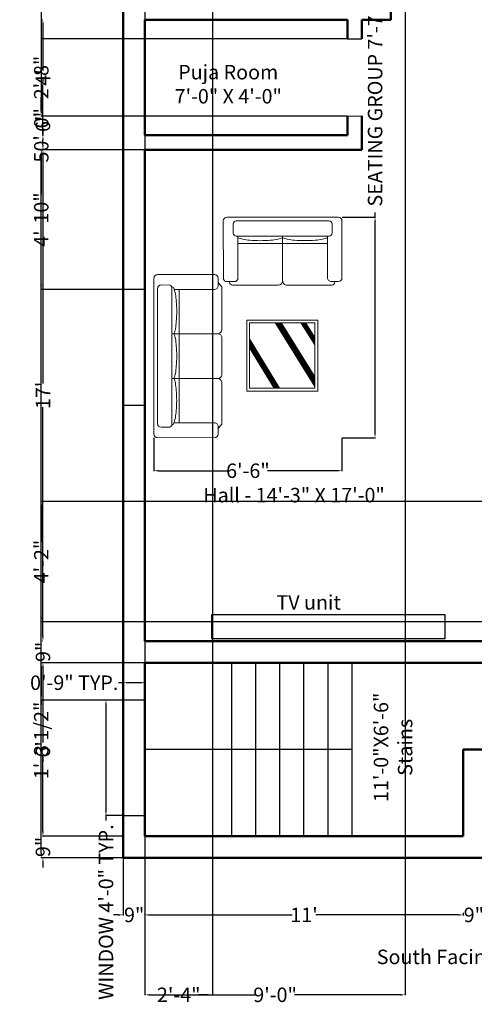
# Model space of a CAD drawing. Units: inches. Extents: x 35 to 505, y 81 to 785.
# Tile 1 of 3: x 35 to 224, y 86 to 495. Entities that reach past the tile are written whole.
import ezdxf

# ---------------------------------------------------------------- set-up
doc = ezdxf.new("R2010")
doc.units = ezdxf.units.IN
doc.header["$MEASUREMENT"] = 0
for name, color, linetype, lineweight in [('A-ANNO-DIMS', 2, 'Continuous', 13), ('A-ANNO-TEXT', 7, 'Continuous', 18), ('A-AREA-IDEN', 7, 'Continuous', 20), ('A-DOOR', 3, 'Continuous', 30), ('A-FLOR-CASE', 8, 'Continuous', 25), ('A-FLOR-STRS', 7, 'Continuous', 25), ('A-FURN', 6, 'Continuous', 18), ('A-GLAZ', 4, 'Continuous', 25), ('A-WALL', 7, 'Continuous', 50)]:
    doc.layers.add(name, color=color, linetype=linetype, lineweight=lineweight)
doc.styles.get("Standard").update_dxf_attribs({"font": 'arial.ttf'})
doc.dimstyles.get("Standard").update_dxf_attribs({"dimtxt": 6, "dimasz": 2, "dimexe": 0.18, "dimexo": 0.0625, "dimgap": 0.09, "dimtad": 0, "dimdec": 0, "dimzin": 0, "dimdsep": 46, "dimlunit": 4, "dimtxsty": 'Standard', "dimcen": 0.09, "dimadec": 0, "dimazin": 0, "dimtfac": 1, "dimtdec": 0, "dimtofl": 0, "dimtmove": 0, "dimatfit": 3, "dimfxl": 1, "dimtolj": 1, "dimtzin": 0, "dimarcsym": 0})

# ---------------------------------------------------------------- blocks, each defined once
blk = doc.blocks.new('*D1')
at = {"layer": 'A-ANNO-DIMS', "color": 0, "lineweight": -2, "transparency": 16777216}
for p, q in [((44.71, 158.11), (44.71, 160.11)), ((77.99, 156.11), (44.53, 156.11)), ((44.65, 147.11), (44.53, 147.11)), ((44.71, 145.11), (44.71, 143.11))]:
    blk.add_line(p, q, dxfattribs=at)
at = {"layer": 'A-ANNO-DIMS', "color": 0, "transparency": 16777216}
for points in [[(44.38, 158.11), (45.04, 158.11), (44.71, 156.11)], [(44.38, 145.11), (45.04, 145.11), (44.71, 147.11)]]:
    blk.add_solid(points, dxfattribs=at)
at = {"layer": 'Defpoints', "color": 0, "transparency": 16777216}
for p in [(44.71, 156.11), (78.06, 156.11), (44.71, 147.11)]:
    blk.add_point(p, dxfattribs=at)
at = {"layer": 'A-ANNO-DIMS', "color": 0, "transparency": 16777216, "insert": (44.71, 151.61), "char_height": 6, "attachment_point": 5, "rotation": 90}
blk.add_mtext('\\A1;9"', dxfattribs=at)
blk = doc.blocks.new('*D2')
at = {"layer": 'A-ANNO-DIMS', "color": 0, "lineweight": -2, "transparency": 16777216}
for p, q in [((44.65, 228.11), (44.53, 228.11)), ((44.71, 226.11), (44.71, 194.98)), ((44.71, 158.11), (44.71, 189.24)), ((44.77, 156.11), (44.89, 156.11))]:
    blk.add_line(p, q, dxfattribs=at)
at = {"layer": 'A-ANNO-DIMS', "color": 0, "transparency": 16777216}
for points in [[(44.38, 226.11), (45.04, 226.11), (44.71, 228.11)], [(44.38, 158.11), (45.04, 158.11), (44.71, 156.11)]]:
    blk.add_solid(points, dxfattribs=at)
at = {"layer": 'Defpoints', "color": 0, "transparency": 16777216}
for p in [(44.71, 228.11), (44.71, 228.11), (44.71, 156.11)]:
    blk.add_point(p, dxfattribs=at)
at = {"layer": 'A-ANNO-DIMS', "color": 0, "transparency": 16777216, "insert": (44.71, 192.11), "char_height": 6, "attachment_point": 5, "rotation": 90}
blk.add_mtext("\\A1;6'", dxfattribs=at)
blk = doc.blocks.new('*D3')
at = {"layer": 'A-ANNO-DIMS', "color": 0, "lineweight": -2, "transparency": 16777216}
for p, q in [((44.71, 239.11), (44.71, 241.11)), ((44.65, 237.11), (44.53, 237.11)), ((44.65, 228.11), (44.53, 228.11)), ((44.71, 226.11), (44.71, 224.11))]:
    blk.add_line(p, q, dxfattribs=at)
at = {"layer": 'A-ANNO-DIMS', "color": 0, "transparency": 16777216}
for points in [[(44.38, 239.11), (45.04, 239.11), (44.71, 237.11)], [(44.38, 226.11), (45.04, 226.11), (44.71, 228.11)]]:
    blk.add_solid(points, dxfattribs=at)
at = {"layer": 'Defpoints', "color": 0, "transparency": 16777216}
for p in [(44.71, 237.11), (44.71, 237.11), (44.71, 228.11)]:
    blk.add_point(p, dxfattribs=at)
at = {"layer": 'A-ANNO-DIMS', "color": 0, "transparency": 16777216, "insert": (44.71, 232.61), "char_height": 6, "attachment_point": 5, "rotation": 90}
blk.add_mtext('\\A1;9"', dxfattribs=at)
blk = doc.blocks.new('*D4')
at = {"layer": 'A-ANNO-DIMS', "color": 0, "lineweight": -2, "transparency": 16777216}
for p, q in [((44.65, 441.11), (44.53, 441.11)), ((44.71, 439.11), (44.71, 344.01)), ((44.71, 239.11), (44.71, 334.21)), ((44.65, 237.11), (44.53, 237.11))]:
    blk.add_line(p, q, dxfattribs=at)
at = {"layer": 'A-ANNO-DIMS', "color": 0, "transparency": 16777216}
for points in [[(44.38, 439.11), (45.04, 439.11), (44.71, 441.11)], [(44.38, 239.11), (45.04, 239.11), (44.71, 237.11)]]:
    blk.add_solid(points, dxfattribs=at)
at = {"layer": 'Defpoints', "color": 0, "transparency": 16777216}
for p in [(44.71, 441.11), (44.71, 441.11), (44.71, 237.11)]:
    blk.add_point(p, dxfattribs=at)
at = {"layer": 'A-ANNO-DIMS', "color": 0, "transparency": 16777216, "insert": (44.71, 339.11), "char_height": 6, "attachment_point": 5, "rotation": 90}
blk.add_mtext("\\A1;17'", dxfattribs=at)
blk = doc.blocks.new('*D5')
at = {"layer": 'A-ANNO-DIMS', "color": 0, "lineweight": -2, "transparency": 16777216}
for p, q in [((44.65, 447.11), (44.53, 447.11)), ((44.71, 447.11), (44.71, 449.11)), ((44.71, 443.11), (44.71, 445.11)), ((44.65, 441.11), (44.53, 441.11))]:
    blk.add_line(p, q, dxfattribs=at)
at = {"layer": 'A-ANNO-DIMS', "color": 0, "transparency": 16777216}
for points in [[(44.38, 445.11), (45.04, 445.11), (44.71, 447.11)], [(44.38, 443.11), (45.04, 443.11), (44.71, 441.11)]]:
    blk.add_solid(points, dxfattribs=at)
at = {"layer": 'Defpoints', "color": 0, "transparency": 16777216}
for p in [(44.71, 447.11), (44.71, 447.11), (44.71, 441.11)]:
    blk.add_point(p, dxfattribs=at)
at = {"layer": 'A-ANNO-DIMS', "color": 0, "transparency": 16777216, "insert": (44.71, 452.66), "char_height": 6, "attachment_point": 5, "rotation": 90}
blk.add_mtext('\\A1;6"', dxfattribs=at)
blk = doc.blocks.new('*D6')
at = {"layer": 'A-ANNO-DIMS', "color": 0, "lineweight": -2, "transparency": 16777216}
for p, q in [((44.65, 495.11), (44.53, 495.11)), ((44.71, 493.11), (44.71, 474.08)), ((44.71, 449.11), (44.71, 468.14)), ((44.71, 447.11), (44.89, 447.11))]:
    blk.add_line(p, q, dxfattribs=at)
at = {"layer": 'A-ANNO-DIMS', "color": 0, "transparency": 16777216}
for points in [[(44.38, 493.11), (45.04, 493.11), (44.71, 495.11)], [(44.38, 449.11), (45.04, 449.11), (44.71, 447.11)]]:
    blk.add_solid(points, dxfattribs=at)
at = {"layer": 'Defpoints', "color": 0, "transparency": 16777216}
for p in [(44.71, 495.11), (44.71, 495.11), (44.65, 447.11)]:
    blk.add_point(p, dxfattribs=at)
at = {"layer": 'A-ANNO-DIMS', "color": 0, "transparency": 16777216, "insert": (44.71, 471.11), "char_height": 6, "attachment_point": 5, "rotation": 90}
blk.add_mtext("\\A1;4'", dxfattribs=at)
blk = doc.blocks.new('*D17')
at = {"layer": 'A-ANNO-DIMS', "color": 0, "lineweight": -2, "transparency": 16777216}
for p, q in [((78.06, 147.05), (78.06, 123.2)), ((76.06, 123.38), (74.06, 123.38)), ((87.06, 124.18), (87.06, 123.2)), ((89.06, 123.38), (91.06, 123.38))]:
    blk.add_line(p, q, dxfattribs=at)
at = {"layer": 'A-ANNO-DIMS', "color": 0, "transparency": 16777216}
for points in [[(76.06, 123.71), (76.06, 123.04), (78.06, 123.38)], [(89.06, 123.71), (89.06, 123.04), (87.06, 123.38)]]:
    blk.add_solid(points, dxfattribs=at)
at = {"layer": 'Defpoints', "color": 0, "transparency": 16777216}
for p in [(78.06, 147.11), (87.06, 124.25), (87.06, 123.38)]:
    blk.add_point(p, dxfattribs=at)
at = {"layer": 'A-ANNO-DIMS', "color": 0, "transparency": 16777216, "insert": (82.56, 123.38), "char_height": 6, "attachment_point": 5}
blk.add_mtext('\\A1;9"', dxfattribs=at)
blk = doc.blocks.new('*D18')
at = {"layer": 'A-ANNO-DIMS', "color": 0, "lineweight": -2, "transparency": 16777216}
for p, q in [((87.06, 123.44), (87.06, 123.56)), ((89.06, 123.38), (148.16, 123.38)), ((217.06, 123.38), (157.96, 123.38)), ((219.06, 124.18), (219.06, 123.2))]:
    blk.add_line(p, q, dxfattribs=at)
at = {"layer": 'A-ANNO-DIMS', "color": 0, "transparency": 16777216}
for points in [[(89.06, 123.71), (89.06, 123.04), (87.06, 123.38)], [(217.06, 123.71), (217.06, 123.04), (219.06, 123.38)]]:
    blk.add_solid(points, dxfattribs=at)
at = {"layer": 'Defpoints', "color": 0, "transparency": 16777216}
for p in [(87.06, 123.38), (219.06, 124.25), (219.06, 123.38)]:
    blk.add_point(p, dxfattribs=at)
at = {"layer": 'A-ANNO-DIMS', "color": 0, "transparency": 16777216, "insert": (153.06, 123.38), "char_height": 6, "attachment_point": 5}
blk.add_mtext("\\A1;11'", dxfattribs=at)
blk = doc.blocks.new('*D19')
at = {"layer": 'A-ANNO-DIMS', "color": 0, "lineweight": -2, "transparency": 16777216}
for p, q in [((217.06, 123.38), (215.06, 123.38)), ((219.06, 124.18), (219.06, 123.2)), ((228.06, 124.18), (228.06, 123.2)), ((230.06, 123.38), (232.06, 123.38))]:
    blk.add_line(p, q, dxfattribs=at)
at = {"layer": 'A-ANNO-DIMS', "color": 0, "transparency": 16777216}
for points in [[(217.06, 123.71), (217.06, 123.04), (219.06, 123.38)], [(230.06, 123.71), (230.06, 123.04), (228.06, 123.38)]]:
    blk.add_solid(points, dxfattribs=at)
at = {"layer": 'Defpoints', "color": 0, "transparency": 16777216}
for p in [(219.06, 124.25), (219.06, 123.38), (228.06, 124.25)]:
    blk.add_point(p, dxfattribs=at)
at = {"layer": 'A-ANNO-DIMS', "color": 0, "transparency": 16777216, "insert": (223.56, 123.38), "char_height": 6, "attachment_point": 5}
blk.add_mtext('\\A1;9"', dxfattribs=at)
blk = doc.blocks.new('sofa')
for p, q in [((639.58, 1159.03, -275.77), (639.59, 1135.36, -275.77)), ((687.29, 1160.58, -275.77), (641.12, 1160.57, -275.77)), ((643.7, 1157.8, -275.77), (643.7, 1153.98, -275.77)), ((683.48, 1159.04, -275.77), (644.93, 1159.03, -275.77)), ((684.72, 1154, -275.77), (684.72, 1157.81, -275.77)), ((688.83, 1159.05, -275.77), (688.84, 1135.38, -275.77)), ((683.49, 1152.76, -275.77), (644.93, 1152.75, -275.77)), ((645.66, 1152.75, -275.77), (645.67, 1135.38, -275.77)), ((682.84, 1149.69, -275.77), (645.66, 1149.67, -275.77)), ((664.21, 1152.76, -275.77), (664.21, 1139.01, -275.77)), ((682.84, 1152.76, -275.77), (682.85, 1135.38, -275.77)), ((635.91, 1136.75, -275.77), (612.28, 1136.74, -275.77)), ((664.21, 1139.01, -275.77), (664.21, 1134.22, -275.77)), ((610.74, 1070.59, -275.77), (610.74, 1135.2, -275.77)), ((637.45, 1132.13, -275.77), (637.45, 1135.21, -275.77)), ((637.45, 1133.47, -275.77), (638.98, 1131.62, -275.77)), ((642.24, 1133.83, -275.77), (641.13, 1133.83, -275.77)), ((642.09, 1133.83, -275.77), (644.13, 1133.84, -275.77)), ((642.2, 1133.83, -275.77), (642.2, 1133.59, -275.77)), ((683.13, 1134.5, -275.77), (683.11, 1134.48, -275.77)), ((687.3, 1133.84, -275.77), (684.39, 1133.84, -275.77)), ((685.84, 1133.84, -275.77), (685.84, 1133.61, -275.77)), ((612.28, 1074.89, -275.77), (612.28, 1130.89, -275.77)), ((613.82, 1132.43, -275.77), (616.9, 1132.44, -275.77)), ((618.26, 1074.18, -275.77), (618.28, 1131.82, -275.77)), ((618.99, 1130.59, -275.77), (619.06, 1130.59, -275.77)), ((635.91, 1130.6, -275.77), (619.16, 1130.59, -275.77)), ((621.21, 1075.35, -275.77), (621.23, 1130.5, -275.77)), ((638.98, 1131.62, -275.77), (638.97, 1113.98, -275.77)), ((662.37, 1132.37, -275.77), (643.43, 1132.36, -275.77)), ((684.61, 1132.38, -275.77), (666.06, 1132.37, -275.77)), ((678.79, 1117.86, -275.77), (649.3, 1117.86, -275.77)), ((649.3, 1117.86, -275.77), (649.3, 1088.37, -275.77)), ((677.59, 1116.66, -275.77), (650.5, 1116.66, -275.77)), ((650.5, 1116.66, -275.77), (650.5, 1089.57, -275.77)), ((677.59, 1090.31, -275.77), (661.29, 1116.65, -275.77)), ((677.59, 1090.75, -275.77), (661.56, 1116.65, -275.77)), ((677.59, 1091.19, -275.77), (661.83, 1116.65, -275.77)), ((677.59, 1091.63, -275.77), (662.1, 1116.65, -275.77)), ((677.59, 1092.07, -275.77), (662.37, 1116.65, -275.77)), ((677.59, 1092.5, -275.77), (662.64, 1116.65, -275.77)), ((677.59, 1092.94, -275.77), (662.91, 1116.65, -275.77)), ((677.59, 1093.38, -275.77), (663.18, 1116.65, -275.77)), ((677.59, 1093.82, -275.77), (663.45, 1116.65, -275.77)), ((677.59, 1094.25, -275.77), (663.73, 1116.65, -275.77)), ((671.89, 1116.65, -275.77), (677.59, 1107.55, -275.77)), ((672.16, 1116.65, -275.77), (677.59, 1107.99, -275.77)), ((672.44, 1116.65, -275.77), (677.59, 1108.42, -275.77)), ((672.71, 1116.65, -275.77), (677.59, 1108.85, -275.77)), ((672.98, 1116.65, -275.77), (677.59, 1109.29, -275.77)), ((673.25, 1116.65, -275.77), (677.59, 1109.72, -275.77)), ((673.52, 1116.65, -275.77), (677.59, 1110.15, -275.77)), ((673.79, 1116.65, -275.77), (677.59, 1110.58, -275.77)), ((677.59, 1089.57, -275.77), (677.59, 1116.66, -275.77)), ((678.79, 1088.37, -275.77), (678.79, 1117.86, -275.77)), ((618.28, 1112.14, -275.77), (637.43, 1112.13, -275.77)), ((638.96, 1095.2, -275.77), (638.97, 1110.59, -275.77)), ((650.5, 1110.11, -275.77), (662.96, 1089.55, -275.77)), ((650.5, 1109.58, -275.77), (662.64, 1089.55, -275.77)), ((650.5, 1109.04, -275.77), (662.31, 1089.55, -275.77)), ((650.5, 1108.5, -275.77), (661.99, 1089.55, -275.77)), ((650.5, 1107.97, -275.77), (661.66, 1089.55, -275.77)), ((650.5, 1107.43, -275.77), (661.34, 1089.55, -275.77)), ((650.5, 1106.9, -275.77), (661.01, 1089.55, -275.77)), ((650.5, 1106.36, -275.77), (660.69, 1089.55, -275.77)), ((618.27, 1093.67, -275.77), (637.43, 1093.66, -275.77)), ((638.96, 1074.67, -275.77), (638.96, 1091.81, -275.77)), ((649.3, 1088.37, -275.77), (678.79, 1088.37, -275.77)), ((650.5, 1089.57, -275.77), (677.59, 1089.57, -275.77)), ((613.82, 1073.35, -275.77), (616.9, 1073.35, -275.77)), ((618.94, 1075.18, -275.77), (635.87, 1075.17, -275.77)), ((618.99, 1075.2, -275.77), (619.06, 1075.2, -275.77)), ((637.43, 1072.82, -275.77), (638.96, 1074.67, -275.77)), ((637.45, 1073.65, -275.77), (637.45, 1070.58, -275.77)), ((635.91, 1069.04, -275.77), (612.28, 1069.05, -275.77))]:
    blk.add_line(p, q)
for centre, radius, start, end in [((641.12, 1159.03, -275.77), 1.54, 90.0228, 180.0228), ((644.93, 1157.8, -275.77), 1.23, 90.0228, 180.0228), ((683.48, 1157.81, -275.77), 1.23, 0.0228, 90.0228), ((687.29, 1159.04, -275.77), 1.54, 0.0228, 90.0228), ((644.93, 1153.98, -275.77), 1.23, 180.0228, 270.0228), ((683.49, 1154, -275.77), 1.23, 270.0228, 0.0228), ((649.8, 1162.3, -275.77), 11.06, 248.0125, 258.4967), ((652.86, 1177.35, -275.77), 26.42, 258.4967, 265.1945), ((654.91, 1201.65, -275.77), 50.81, 265.1945, 270.0228), ((654.91, 1201.65, -275.77), 50.81, 270.0228, 274.8511), ((656.97, 1177.35, -275.77), 26.42, 274.8511, 281.549), ((660.04, 1162.3, -275.77), 11.06, 281.549, 292.4094), ((668.32, 1162.3, -275.77), 11.06, 247.6363, 258.4967), ((671.38, 1177.35, -275.77), 26.42, 258.4967, 265.1945), ((673.43, 1201.66, -275.77), 50.81, 265.1945, 270.0228), ((673.43, 1201.66, -275.77), 50.81, 270.0228, 274.8511), ((675.49, 1177.36, -275.77), 26.42, 274.8511, 281.549), ((678.56, 1162.31, -275.77), 11.06, 281.549, 292.7616), ((641.13, 1135.37, -275.77), 1.54, 180.0228, 270.0228), ((643.43, 1133.59, -275.77), 1.23, 180.0228, 270.0228), ((644.13, 1135.37, -275.77), 1.54, 270.0228, 0.0228), ((662.37, 1134.22, -275.77), 1.85, 270.0228, 0.0228), ((666.06, 1134.22, -275.77), 1.85, 180.0228, 270.0228), ((684.39, 1135.38, -275.77), 1.54, 180.0228, 270.0228), ((684.61, 1133.61, -275.77), 1.23, 270.0228, 0.0228), ((687.3, 1135.38, -275.77), 1.54, 270.0228, 0.0228)]:
    blk.add_arc(centre, radius, start, end)
for centre, major_axis, start_param, end_param in [((612.28, 1135.2, -275.77), (1.09, -1.09), 2.356593, 3.927389), ((635.91, 1135.21, -275.77), (-1.09, -1.09), 2.356593, 3.927389), ((613.82, 1130.9, -275.77), (1.09, -1.09), 2.356593, 3.927389), ((616.9, 1130.9, -275.77), (1.09, -1.09), 1.162634, 2.356593), ((618.35, 1131.11, -275.77), (-0.395, -0.395), 2.777055, 3.922193), ((608.13, 1126.54, -275.77), (8.31, -8.31), 0.968514, 1.206259), ((591.77, 1123.51, -275.77), (-20.08, -20.08), 2.432524, 2.53931), ((635.91, 1132.13, -275.77), (1.09, -1.09), -0.785, 0.785796), ((565.27, 1121.49, -275.77), (-38.87, -38.87), 2.355796, 2.432524), ((565.27, 1121.49, -275.77), (38.87, -38.87), 0.708272, 0.785), ((591.76, 1119.44, -275.77), (20.08, -20.08), 0.601486, 0.708272), ((608.13, 1116.39, -275.77), (-8.31, -8.31), 1.988696, 2.172282), ((608.13, 1108.03, -275.77), (-8.31, -8.31), 2.53931, 2.722897), ((637.13, 1113.98, -275.77), (-1.31, -1.31), 0.785, 2.355796), ((637.43, 1110.59, -275.77), (-1.09, -1.09), 2.355796, 3.926593), ((591.76, 1105, -275.77), (-20.08, -20.08), 2.432524, 2.53931), ((565.26, 1102.97, -275.77), (-38.87, -38.87), 2.355796, 2.432524), ((565.26, 1102.97, -275.77), (38.87, -38.87), 0.708272, 0.785), ((608.12, 1097.88, -275.77), (8.31, -8.31), 0.417899, 0.601486), ((591.76, 1100.92, -275.77), (-20.08, -20.08), 2.172282, 2.279068), ((608.12, 1089.61, -275.77), (8.31, -8.31), 0.968514, 1.1521), ((591.75, 1086.58, -275.77), (20.08, -20.08), 0.861728, 0.968514), ((637.12, 1091.81, -275.77), (-1.31, -1.31), 2.355796, 3.926593), ((637.43, 1095.2, -275.77), (1.09, -1.09), -0.785796, 0.785), ((565.25, 1084.55, -275.77), (-38.87, -38.87), 2.355796, 2.432524), ((565.25, 1084.55, -275.77), (38.87, -38.87), 0.708272, 0.785), ((591.75, 1082.51, -275.77), (-20.08, -20.08), 2.172282, 2.279068), ((608.12, 1079.46, -275.77), (8.31, -8.31), 0.363741, 0.601486), ((613.82, 1074.89, -275.77), (-1.09, -1.09), 5.497389, 7.068185), ((616.9, 1074.89, -275.77), (-1.09, -1.09), 0.785, 1.978958), ((618.32, 1074.88, -275.77), (-0.395, -0.395), 0.79242, 1.934537), ((635.91, 1073.65, -275.77), (-1.09, -1.09), 2.355796, 3.926593), ((612.28, 1070.59, -275.77), (-1.09, -1.09), 5.497389, 7.068185), ((635.91, 1070.58, -275.77), (1.09, -1.09), -0.785796, 0.785)]:
    blk.add_ellipse(centre, major_axis=major_axis, ratio=1, start_param=start_param, end_param=end_param)
blk = doc.blocks.new('WIN-48-JAMBS')
for p, q in [((9, 48), (0, 48)), ((0, 0), (9, 0))]:
    blk.add_line(p, q)
blk = doc.blocks.new('*D44')
at = {"layer": 'A-ANNO-DIMS', "color": 0, "lineweight": -2, "transparency": 16777216}
for p, q in [((77.99, 212.6), (70.68, 212.6)), ((70.86, 210.6), (70.86, 166.6)), ((77.99, 164.6), (70.68, 164.6)), ((70.86, 164.6), (70.86, 162.6))]:
    blk.add_line(p, q, dxfattribs=at)
at = {"layer": 'A-ANNO-DIMS', "color": 0, "transparency": 16777216}
for points in [[(70.52, 210.6), (71.19, 210.6), (70.86, 212.6)], [(70.52, 166.6), (71.19, 166.6), (70.86, 164.6)]]:
    blk.add_solid(points, dxfattribs=at)
at = {"layer": 'Defpoints', "color": 0, "transparency": 16777216}
for p in [(78.06, 212.6), (70.86, 164.6), (78.06, 164.6)]:
    blk.add_point(p, dxfattribs=at)
at = {"layer": 'A-ANNO-DIMS', "color": 0, "transparency": 16777216, "insert": (70.86, 124.55), "char_height": 6, "attachment_point": 5, "rotation": 90}
blk.add_mtext('\\A1;WINDOW 4\'-0" TYP.', dxfattribs=at)
blk = doc.blocks.new('*D45')
at = {"layer": 'A-ANNO-DIMS', "color": 0, "lineweight": -2, "transparency": 16777216}
for p, q in [((78.06, 219.8), (76.06, 219.8)), ((78.06, 212.66), (78.06, 219.98)), ((85.06, 219.8), (80.06, 219.8)), ((87.06, 212.66), (87.06, 219.98))]:
    blk.add_line(p, q, dxfattribs=at)
at = {"layer": 'A-ANNO-DIMS', "color": 0, "transparency": 16777216}
for points in [[(80.06, 220.14), (80.06, 219.47), (78.06, 219.8)], [(85.06, 220.14), (85.06, 219.47), (87.06, 219.8)]]:
    blk.add_solid(points, dxfattribs=at)
at = {"layer": 'Defpoints', "color": 0, "transparency": 16777216}
for p in [(78.06, 219.8), (78.06, 212.6), (87.06, 212.6)]:
    blk.add_point(p, dxfattribs=at)
at = {"layer": 'A-ANNO-DIMS', "color": 0, "transparency": 16777216, "insert": (57.68, 219.8), "char_height": 6, "attachment_point": 5}
blk.add_mtext('\\A1;0\'-9" TYP.', dxfattribs=at)
blk = doc.blocks.new('*D50')
at = {"layer": 'A-ANNO-DIMS', "color": 0, "lineweight": -2, "transparency": 16777216}
for p, q in [((168.89, 413.09), (182.74, 413.09)), ((182.56, 413.09), (182.56, 415.09)), ((182.56, 323.55), (182.56, 411.09)), ((168.89, 321.55), (182.74, 321.55))]:
    blk.add_line(p, q, dxfattribs=at)
at = {"layer": 'A-ANNO-DIMS', "color": 0, "transparency": 16777216}
for points in [[(182.23, 411.09), (182.89, 411.09), (182.56, 413.09)], [(182.23, 323.55), (182.89, 323.55), (182.56, 321.55)]]:
    blk.add_solid(points, dxfattribs=at)
at = {"layer": 'Defpoints', "color": 0, "transparency": 16777216}
for p in [(168.83, 413.09), (182.56, 413.09), (168.83, 321.55)]:
    blk.add_point(p, dxfattribs=at)
at = {"layer": 'A-ANNO-DIMS', "color": 0, "transparency": 16777216, "insert": (182.56, 466.23), "char_height": 6, "attachment_point": 5, "rotation": 90}
blk.add_mtext('\\A1;SEATING GROUP 7\'-7 1/2"', dxfattribs=at)
blk = doc.blocks.new('*D51')
at = {"layer": 'A-ANNO-DIMS', "color": 0, "lineweight": -2, "transparency": 16777216}
for p, q in [((90.73, 321.49), (90.73, 307.64)), ((168.83, 321.49), (168.83, 307.64)), ((92.73, 307.82), (121.7, 307.82)), ((166.83, 307.82), (137.86, 307.82))]:
    blk.add_line(p, q, dxfattribs=at)
at = {"layer": 'A-ANNO-DIMS', "color": 0, "transparency": 16777216}
for points in [[(92.73, 308.15), (92.73, 307.48), (90.73, 307.82)], [(166.83, 308.15), (166.83, 307.48), (168.83, 307.82)]]:
    blk.add_solid(points, dxfattribs=at)
at = {"layer": 'Defpoints', "color": 0, "transparency": 16777216}
for p in [(90.73, 321.55), (168.83, 321.55), (168.83, 307.82)]:
    blk.add_point(p, dxfattribs=at)
at = {"layer": 'A-ANNO-DIMS', "color": 0, "transparency": 16777216, "insert": (129.78, 307.82), "char_height": 6, "attachment_point": 5}
blk.add_mtext('\\A1;6\'-6"', dxfattribs=at)
blk = doc.blocks.new('*D53')
at = {"layer": 'A-ANNO-DIMS', "color": 0, "lineweight": -2, "transparency": 16777216}
for p, q in [((77.99, 747.11), (43.83, 747.11)), ((44.01, 745.11), (44.01, 457.5)), ((44.01, 149.11), (44.01, 436.71)), ((77.99, 147.11), (43.83, 147.11))]:
    blk.add_line(p, q, dxfattribs=at)
at = {"layer": 'A-ANNO-DIMS', "color": 0, "transparency": 16777216}
for points in [[(43.67, 745.11), (44.34, 745.11), (44.01, 747.11)], [(43.67, 149.11), (44.34, 149.11), (44.01, 147.11)]]:
    blk.add_solid(points, dxfattribs=at)
at = {"layer": 'Defpoints', "color": 0, "transparency": 16777216}
for p in [(44.01, 747.11), (78.06, 747.11), (78.06, 147.11)]:
    blk.add_point(p, dxfattribs=at)
at = {"layer": 'A-ANNO-DIMS', "color": 0, "transparency": 16777216, "insert": (44.01, 447.11), "char_height": 6, "attachment_point": 5, "rotation": 90}
blk.add_mtext('\\A1;50\'-0"', dxfattribs=at)
blk = doc.blocks.new('*D54')
at = {"layer": 'A-ANNO-DIMS', "color": 0, "lineweight": -2, "transparency": 16777216}
for p, q in [((87.06, 738.05), (87.06, 90.02)), ((195.06, 738.05), (195.06, 90.02)), ((89.06, 90.2), (132.99, 90.2)), ((193.06, 90.2), (149.12, 90.2))]:
    blk.add_line(p, q, dxfattribs=at)
at = {"layer": 'A-ANNO-DIMS', "color": 0, "transparency": 16777216}
for points in [[(89.06, 90.53), (89.06, 89.86), (87.06, 90.2)], [(193.06, 90.53), (193.06, 89.86), (195.06, 90.2)]]:
    blk.add_solid(points, dxfattribs=at)
at = {"layer": 'Defpoints', "color": 0, "transparency": 16777216}
for p in [(87.06, 738.11), (195.06, 738.11), (195.06, 90.2)]:
    blk.add_point(p, dxfattribs=at)
at = {"layer": 'A-ANNO-DIMS', "color": 0, "transparency": 16777216, "insert": (141.06, 90.2), "char_height": 6, "attachment_point": 5}
blk.add_mtext('\\A1;9\'-0"', dxfattribs=at)
blk = doc.blocks.new('*D56')
at = {"layer": 'A-ANNO-DIMS', "color": 0, "lineweight": -2, "transparency": 16777216}
for p, q in [((86.99, 441.11), (43.83, 441.11)), ((44.01, 439.11), (44.01, 422.61)), ((44.01, 385.09), (44.01, 401.58)), ((86.99, 383.09), (43.83, 383.09))]:
    blk.add_line(p, q, dxfattribs=at)
at = {"layer": 'A-ANNO-DIMS', "color": 0, "transparency": 16777216}
for points in [[(43.67, 439.11), (44.34, 439.11), (44.01, 441.11)], [(43.67, 385.09), (44.34, 385.09), (44.01, 383.09)]]:
    blk.add_solid(points, dxfattribs=at)
at = {"layer": 'Defpoints', "color": 0, "transparency": 16777216}
for p in [(87.06, 441.11), (44.01, 383.09), (87.06, 383.09)]:
    blk.add_point(p, dxfattribs=at)
at = {"layer": 'A-ANNO-DIMS', "color": 0, "transparency": 16777216, "insert": (44.01, 412.1), "char_height": 6, "attachment_point": 5, "rotation": 90}
blk.add_mtext('\\A1;4\'-10"', dxfattribs=at)
blk = doc.blocks.new('*D57')
at = {"layer": 'A-ANNO-DIMS', "color": 0, "lineweight": -2, "transparency": 16777216}
for p, q in [((86.99, 228.11), (43.83, 228.11)), ((44.01, 226.11), (44.01, 214.6)), ((86.99, 212.6), (43.83, 212.6)), ((44.01, 212.6), (44.01, 210.6))]:
    blk.add_line(p, q, dxfattribs=at)
at = {"layer": 'A-ANNO-DIMS', "color": 0, "transparency": 16777216}
for points in [[(43.67, 226.11), (44.34, 226.11), (44.01, 228.11)], [(43.67, 214.6), (44.34, 214.6), (44.01, 212.6)]]:
    blk.add_solid(points, dxfattribs=at)
at = {"layer": 'Defpoints', "color": 0, "transparency": 16777216}
for p in [(87.06, 228.11), (44.01, 212.6), (87.06, 212.6)]:
    blk.add_point(p, dxfattribs=at)
at = {"layer": 'A-ANNO-DIMS', "color": 0, "transparency": 16777216, "insert": (44.01, 195.83), "char_height": 6, "attachment_point": 5, "rotation": 90}
blk.add_mtext('\\A1;1\'-3 1/2"', dxfattribs=at)
blk = doc.blocks.new('*D58')
at = {"layer": 'A-ANNO-DIMS', "color": 0, "lineweight": -2, "transparency": 16777216}
for p, q in [((257.99, 295.11), (43.83, 295.11)), ((44.01, 293.11), (44.01, 278.29)), ((44.01, 247.11), (44.01, 261.92)), ((257.99, 245.11), (43.83, 245.11))]:
    blk.add_line(p, q, dxfattribs=at)
at = {"layer": 'A-ANNO-DIMS', "color": 0, "transparency": 16777216}
for points in [[(43.67, 293.11), (44.34, 293.11), (44.01, 295.11)], [(43.67, 247.11), (44.34, 247.11), (44.01, 245.11)]]:
    blk.add_solid(points, dxfattribs=at)
at = {"layer": 'Defpoints', "color": 0, "transparency": 16777216}
for p in [(44.01, 295.11), (258.06, 295.11), (258.06, 245.11)]:
    blk.add_point(p, dxfattribs=at)
at = {"layer": 'A-ANNO-DIMS', "color": 0, "transparency": 16777216, "insert": (44.01, 270.11), "char_height": 6, "attachment_point": 5, "rotation": 90}
blk.add_mtext('\\A1;4\'-2"', dxfattribs=at)
blk = doc.blocks.new('*D61')
at = {"layer": 'A-ANNO-DIMS', "color": 0, "lineweight": -2, "transparency": 16777216}
for p, q in [((87.06, 738.05), (87.06, 90.02)), ((115.06, 738.05), (115.06, 90.02)), ((89.06, 90.2), (92.94, 90.2)), ((113.06, 90.2), (109.17, 90.2))]:
    blk.add_line(p, q, dxfattribs=at)
at = {"layer": 'A-ANNO-DIMS', "color": 0, "transparency": 16777216}
for points in [[(89.06, 90.53), (89.06, 89.86), (87.06, 90.2)], [(113.06, 90.53), (113.06, 89.86), (115.06, 90.2)]]:
    blk.add_solid(points, dxfattribs=at)
at = {"layer": 'Defpoints', "color": 0, "transparency": 16777216}
for p in [(87.06, 738.11), (115.06, 738.11), (115.06, 90.2)]:
    blk.add_point(p, dxfattribs=at)
at = {"layer": 'A-ANNO-DIMS', "color": 0, "transparency": 16777216, "insert": (101.06, 90.2), "char_height": 6, "attachment_point": 5}
blk.add_mtext('\\A1;2\'-4"', dxfattribs=at)
blk = doc.blocks.new('*D64')
at = {"layer": 'A-ANNO-DIMS', "color": 0, "lineweight": -2, "transparency": 16777216}
for p, q in [((170.99, 487.11), (43.83, 487.11)), ((44.01, 485.11), (44.01, 479.22)), ((44.01, 457.11), (44.01, 462.99)), ((170.99, 455.11), (43.83, 455.11))]:
    blk.add_line(p, q, dxfattribs=at)
at = {"layer": 'A-ANNO-DIMS', "color": 0, "transparency": 16777216}
for points in [[(43.67, 485.11), (44.34, 485.11), (44.01, 487.11)], [(43.67, 457.11), (44.34, 457.11), (44.01, 455.11)]]:
    blk.add_solid(points, dxfattribs=at)
at = {"layer": 'Defpoints', "color": 0, "transparency": 16777216}
for p in [(44.01, 487.11), (171.06, 487.11), (171.06, 455.11)]:
    blk.add_point(p, dxfattribs=at)
at = {"layer": 'A-ANNO-DIMS', "color": 0, "transparency": 16777216, "insert": (44.01, 471.11), "char_height": 6, "attachment_point": 5, "rotation": 90}
blk.add_mtext('\\A1;2\'-8"', dxfattribs=at)

msp = doc.modelspace()

# ---------------------------------------------------------------- linework, layer by layer
at = {"layer": 'A-DOOR'}
for p, q in [((171.02, 487.11), (177.06, 487.12)), ((171.06, 455.11), (177.06, 455.12))]:
    msp.add_line(p, q, dxfattribs=at)
at = {"layer": 'A-FLOR-CASE'}
msp.add_lwpolyline([(114.62, 238.12), (211.65, 238.12), (211.65, 248.04), (114.62, 248.04)], close=True, dxfattribs=at)
at = {"layer": 'A-FLOR-STRS'}
for p, q in [((123.06, 156.11), (123.06, 228.11)), ((133.06, 156.11), (133.06, 228.11)), ((143.06, 156.11), (143.06, 228.11)), ((153.06, 156.11), (153.06, 228.11)), ((163.06, 156.11), (163.06, 228.11)), ((173.06, 156.11), (173.06, 228.11)), ((173.06, 192.11), (87.06, 192.11))]:
    msp.add_line(p, q, dxfattribs=at)
at = {"layer": 'A-WALL'}
for p, q in [((78.06, 747.11), (78.06, 147.11)), ((189.06, 501.11), (189.06, 495.11)), ((87.06, 447.11), (87.06, 495.11)), ((171.06, 495.11), (87.06, 495.11)), ((171.06, 495.11), (171.06, 487.11)), ((189.06, 495.11), (177.06, 495.11)), ((177.06, 495.11), (177.06, 487.12)), ((171.06, 455.11), (171.06, 447.11)), ((177.06, 455.12), (177.06, 441.11)), ((171.06, 447.11), (87.06, 447.11)), ((87.06, 237.11), (87.06, 441.11)), ((177.06, 441.11), (87.06, 441.11)), ((258.06, 237.11), (87.06, 237.11)), ((87.06, 156.11), (87.06, 228.11)), ((219.06, 228.11), (87.06, 228.11)), ((312.06, 228.11), (219.06, 228.11)), ((219.06, 192.11), (219.06, 156.11)), ((228.06, 192.11), (219.06, 192.11)), ((219.06, 156.11), (87.06, 156.11)), ((321.06, 147.11), (78.06, 147.11))]:
    msp.add_line(p, q, dxfattribs=at)

# ---------------------------------------------------------------- block references
at = {"layer": 'A-FURN'}
msp.add_blockref('sofa', (-520.01, -747.49, 275.77), dxfattribs=at)
at = {"layer": 'A-GLAZ', "rotation": 180}
for p in [(87.06, 383.09), (87.06, 212.6)]:
    msp.add_blockref('WIN-48-JAMBS', p, dxfattribs=at)

# ---------------------------------------------------------------- texts
at = {"layer": 'A-ANNO-TEXT', "char_height": 6, "attachment_point": 1}
for s, width, insert in [('\\pxqc;TV unit', 50.81, (129.59, 256.14)), ('\\pxqc;South Facing Building - Road', 193.0111, (141.71, 108.95))]:
    msp.add_mtext_dynamic_manual_height_columns(s, width=width, gutter_width=30, heights=[0], dxfattribs=dict(at, insert=insert))
at = {"layer": 'A-AREA-IDEN', "char_height": 6, "attachment_point": 1}
for s, width, insert in [('\\pxqc;Puja Room\\P7\'-0" X 4\'-0"', 80.9997, (81.12, 476.32)), ('\\pxqc;Hall - 14\'-3" X 17\'-0"', 89.3896, (104.23, 300.69))]:
    msp.add_mtext_dynamic_manual_height_columns(s, width=width, gutter_width=30, heights=[0], dxfattribs=dict(at, insert=insert))
at = {"layer": 'A-AREA-IDEN', "insert": (182.02, 126.01), "char_height": 6, "attachment_point": 1, "rotation": 90}
msp.add_mtext_dynamic_manual_height_columns('\\pxqc;11\'-0"X6\'-6"\\PStains', width=133.9079, gutter_width=30, heights=[0], dxfattribs=at)

# ---------------------------------------------------------------- dimensions: what is measured, and where the dimension line sits
at = {"layer": 'A-ANNO-DIMS'}
for base, p1, p2, override, picture, middle in [((44.01, 747.11), (78.06, 147.11), (78.06, 747.11), {"dimdec": 1, "dimlfac": 1, "dimrnd": 0, "dimzin": 1, "dimdsep": 46, "dimlunit": 4, "dimfrac": 2}, '*D53', (44.01, 447.11)), ((44.71, 495.11), (44.65, 447.11), (44.71, 495.11), {"dimclrd": 0, "dimclre": 0, "dimclrt": 0}, '*D6', (44.71, 471.11)), ((44.01, 487.11), (171.06, 455.11), (171.06, 487.11), {"dimdec": 1, "dimlfac": 1, "dimrnd": 0, "dimzin": 1, "dimdsep": 46, "dimlunit": 4, "dimfrac": 2}, '*D64', (44.01, 471.11)), ((44.71, 447.11), (44.71, 441.11), (44.71, 447.11), {"dimclrd": 0, "dimclre": 0, "dimclrt": 0}, '*D5', (44.71, 452.66)), ((44.01, 383.09), (87.06, 441.11), (87.06, 383.09), {"dimdec": 1, "dimlfac": 1, "dimrnd": 0, "dimzin": 1, "dimdsep": 46, "dimlunit": 4, "dimfrac": 2}, '*D56', (44.01, 412.1)), ((44.71, 441.11), (44.71, 237.11), (44.71, 441.11), {"dimclrd": 0, "dimclre": 0, "dimclrt": 0}, '*D4', (44.71, 339.11)), ((44.01, 295.11), (258.06, 245.11), (258.06, 295.11), {"dimdec": 1, "dimlfac": 1, "dimrnd": 0, "dimzin": 1, "dimdsep": 46, "dimlunit": 4, "dimfrac": 2}, '*D58', (44.01, 270.11)), ((44.71, 237.11), (44.71, 228.11), (44.71, 237.11), {"dimclrd": 0, "dimclre": 0, "dimclrt": 0}, '*D3', (44.71, 232.61)), ((44.01, 212.6), (87.06, 228.11), (87.06, 212.6), {"dimdec": 1, "dimlfac": 1, "dimrnd": 0, "dimzin": 1, "dimdsep": 46, "dimlunit": 4, "dimfrac": 2}, '*D57', (44.01, 195.83)), ((44.71, 228.11), (44.71, 156.11), (44.71, 228.11), {"dimclrd": 0, "dimclre": 0, "dimclrt": 0}, '*D2', (44.71, 192.11)), ((44.71, 156.11), (44.71, 147.11), (78.06, 156.11), {"dimclrd": 0, "dimclre": 0, "dimclrt": 0}, '*D1', (44.71, 151.61))]:
    dim = msp.add_linear_dim(base=base, p1=p1, p2=p2, angle=90, dimstyle='Standard', override=override, dxfattribs=at)
    dim.commit()
    dim.dimension.update_dxf_attribs({"geometry": picture, "text_midpoint": middle})
for base, p1, p2, override, picture, middle in [((195.06, 90.2), (87.06, 738.11), (195.06, 738.11), {"dimdec": 1, "dimlfac": 1, "dimrnd": 0, "dimzin": 1, "dimdsep": 46, "dimlunit": 4, "dimfrac": 2}, '*D54', (141.06, 90.2)), ((115.06, 90.2), (87.06, 738.11), (115.06, 738.11), {"dimdec": 1, "dimlfac": 1, "dimrnd": 0, "dimzin": 1, "dimdsep": 46, "dimlunit": 4, "dimfrac": 2}, '*D61', (101.06, 90.2)), ((168.83, 307.82), (90.73, 321.55), (168.83, 321.55), {"dimdec": 1, "dimlfac": 1, "dimrnd": 0, "dimzin": 1, "dimdsep": 46, "dimlunit": 4, "dimfrac": 2}, '*D51', (129.78, 307.82)), ((87.06, 123.38), (78.06, 147.11), (87.06, 124.25), {"dimclrd": 0, "dimclre": 0, "dimclrt": 0}, '*D17', (82.56, 123.38)), ((219.06, 123.38), (87.06, 123.38), (219.06, 124.25), {"dimclrd": 0, "dimclre": 0, "dimclrt": 0}, '*D18', (153.06, 123.38)), ((219.06, 123.38), (228.06, 124.25), (219.06, 124.25), {"dimclrd": 0, "dimclre": 0, "dimclrt": 0}, '*D19', (223.56, 123.38))]:
    dim = msp.add_linear_dim(base=base, p1=p1, p2=p2, dimstyle='Standard', override=override, dxfattribs=at)
    dim.commit()
    dim.dimension.update_dxf_attribs({"geometry": picture, "text_midpoint": middle})
for base, p1, p2, angle, text, picture, middle in [((182.56, 413.09), (168.83, 321.55), (168.83, 413.09), 90, 'SEATING GROUP <>', '*D50', (182.56, 466.23)), ((78.06, 219.8), (87.06, 212.6), (78.06, 212.6), 180, '<> TYP.', '*D45', (57.68, 219.8)), ((70.86, 164.6), (78.06, 212.6), (78.06, 164.6), 270, 'WINDOW <> TYP.', '*D44', (70.86, 124.55))]:
    dim = msp.add_linear_dim(base=base, p1=p1, p2=p2, angle=angle, text=text, dimstyle='Standard', override={"dimdec": 1, "dimlfac": 1, "dimrnd": 0, "dimzin": 1, "dimdsep": 46, "dimlunit": 4, "dimfrac": 2}, dxfattribs=at)
    dim.commit()
    dim.dimension.update_dxf_attribs({"geometry": picture, "text_midpoint": middle})

doc.saveas('drawing.dxf')
